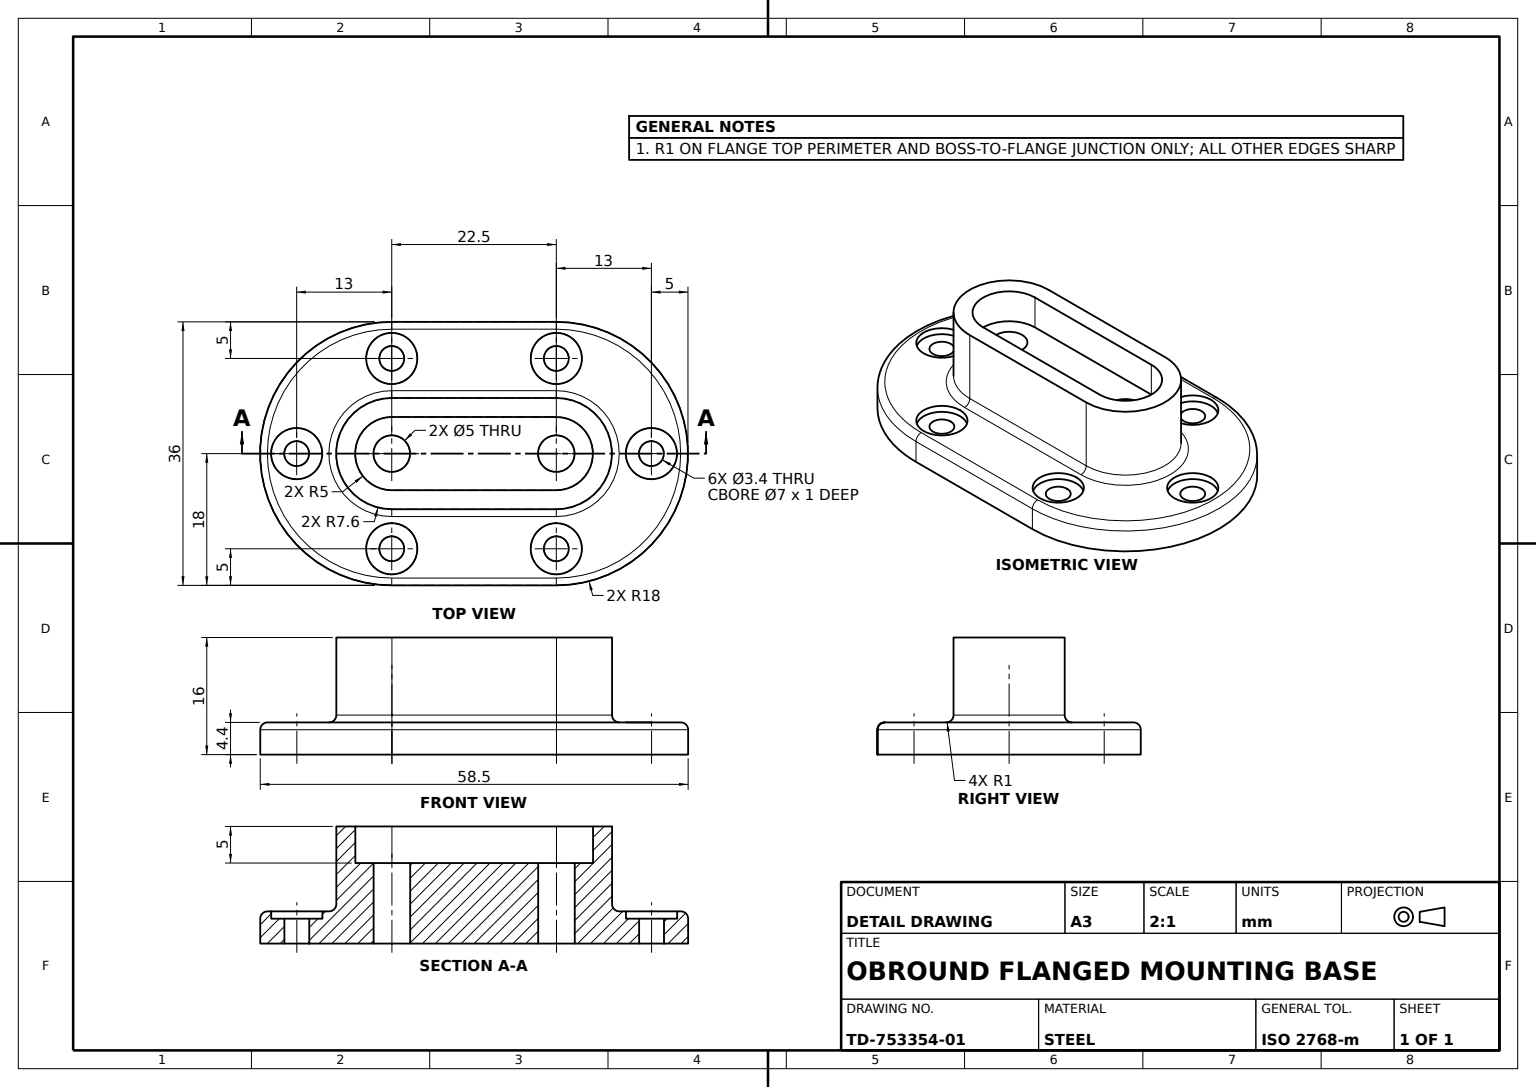
from build123d import *

# Parameters (mm, degrees)
OVAL_BASE_FLANGE_DEPTH           = 4.4
RAISED_OVAL_BOSS_DEPTH           = 11.6
OVAL_POCKET_R5_DEPTH             = 5
COUNTERBORE_SKETCH_R             = 3.5
MOUNTING_HOLE_COUNTERBORES_DEPTH = 1
MOUNTING_HOLES_SKETCH_R          = 1.7
MOUNTING_HOLES_3_4_DEPTH         = 7
THROUGH_SLOT_SKETCH_R            = 2.5
POCKET_THROUGH_SLOT_DEPTH        = 15
BOSS_ROOT_FILLET_R1_R            = 1


with BuildPart() as part:
    # Base Flange Sketch → Oval Base Flange (new body)
    with BuildSketch(Plane(origin=(0, 0, 0), x_dir=(1, 0, 0), z_dir=(0, 1, 0))):
        with BuildLine():
            Line((11.25, -18), (-11.25, -18))
            ThreePointArc((-11.25, -18), (-29.25, 0), (-11.25, 18))
            Line((-11.25, 18), (11.25, 18))
            ThreePointArc((11.25, 18), (29.25, 0), (11.25, -18))
        make_face()
    extrude(amount=OVAL_BASE_FLANGE_DEPTH)

    # Oval Boss Sketch → Raised Oval Boss (add)
    with BuildSketch(Plane(origin=(0, 4.4, 0), x_dir=(1, 0, 0), z_dir=(0, 1, 0))):
        with BuildLine():
            Line((-11.25, 7.6), (11.25, 7.6))
            ThreePointArc((11.25, 7.6), (18.85, 0), (11.25, -7.6))
            Line((11.25, -7.6), (-11.25, -7.6))
            ThreePointArc((-11.25, -7.6), (-18.85, 0), (-11.25, 7.6))
        make_face()
    extrude(amount=RAISED_OVAL_BOSS_DEPTH)

    # Oval Pocket Sketch → Oval Pocket R5 (cut)
    with BuildSketch(Plane(origin=(0, 16, 0), x_dir=(1, 0, 0), z_dir=(0, 1, 0))):
        with BuildLine():
            Line((-11.25, 5), (11.25, 5))
            ThreePointArc((11.25, 5), (16.25, 0), (11.25, -5))
            Line((11.25, -5), (-11.25, -5))
            ThreePointArc((-11.25, -5), (-16.25, 0), (-11.25, 5))
        make_face()
    extrude(amount=-OVAL_POCKET_R5_DEPTH, mode=Mode.SUBTRACT)

    # Counterbore Sketch → Mounting Hole Counterbores (cut)
    with BuildSketch(Plane(origin=(0, 4.4, 0), x_dir=(1, 0, 0), z_dir=(0, 1, 0))):
        with Locations(Location((-11.25, 13, 0), (0, 0, 270))):
            Circle(COUNTERBORE_SKETCH_R)
        with Locations(Location((11.25, 13, 0), (0, 0, 90))):
            Circle(COUNTERBORE_SKETCH_R)
        with Locations(Location((11.25, -13, 0), (0, 0, 270))):
            Circle(COUNTERBORE_SKETCH_R)
        with Locations(Location((-11.25, -13, 0), (0, 0, 90))):
            Circle(COUNTERBORE_SKETCH_R)
        with Locations(Location((-24.25, 0, 0), (0, 0, 270))):
            Circle(COUNTERBORE_SKETCH_R)
        with Locations(Location((24.25, 0, 0), (0, 0, 90))):
            Circle(COUNTERBORE_SKETCH_R)
    extrude(amount=-MOUNTING_HOLE_COUNTERBORES_DEPTH, mode=Mode.SUBTRACT)

    # Mounting Holes Sketch → Mounting Holes Ø3.4 (cut)
    with BuildSketch(Plane(origin=(0, 3.4, 0), x_dir=(1, 0, 0), z_dir=(0, 1, 0))):
        with Locations(Location((-11.25, 13, 0), (0, 0, 270))):
            Circle(MOUNTING_HOLES_SKETCH_R)
        with Locations(Location((11.25, 13, 0), (0, 0, 270))):
            Circle(MOUNTING_HOLES_SKETCH_R)
        with Locations(Location((11.25, -13, 0), (0, 0, 270))):
            Circle(MOUNTING_HOLES_SKETCH_R)
        with Locations(Location((-11.25, -13, 0), (0, 0, 270))):
            Circle(MOUNTING_HOLES_SKETCH_R)
        with Locations(Location((-24.25, 0, 0), (0, 0, 270))):
            Circle(MOUNTING_HOLES_SKETCH_R)
        with Locations(Location((24.25, 0, 0), (0, 0, 270))):
            Circle(MOUNTING_HOLES_SKETCH_R)
    extrude(amount=-MOUNTING_HOLES_3_4_DEPTH, mode=Mode.SUBTRACT)

    # Through Slot Sketch → Pocket Through Slot (cut)
    with BuildSketch(Plane(origin=(0, 11, 0), x_dir=(1, 0, 0), z_dir=(0, 1, 0))):
        with Locations(Location((-11.25, 0, 0), (0, 0, 270))):
            Circle(THROUGH_SLOT_SKETCH_R)
        with Locations(Location((11.25, 0, 0), (0, 0, 270))):
            Circle(THROUGH_SLOT_SKETCH_R)
    extrude(amount=-POCKET_THROUGH_SLOT_DEPTH, mode=Mode.SUBTRACT)

    # Boss Root Fillet R1
    boss_root_fillet_r1_edges = [part.edges().sort_by_distance(p)[0] for p in [
        (-29.25, 4.4, 0),
        (-18.85, 4.4, 0),
        (0, 4.4, 18),
        (0, 4.4, 7.6),
        (18.85, 4.4, 0),
        (0, 4.4, -7.6),
        (29.25, 4.4, 0),
        (0, 4.4, -18),
    ]]
    fillet(boss_root_fillet_r1_edges, radius=BOSS_ROOT_FILLET_R1_R)


solid = part.part
